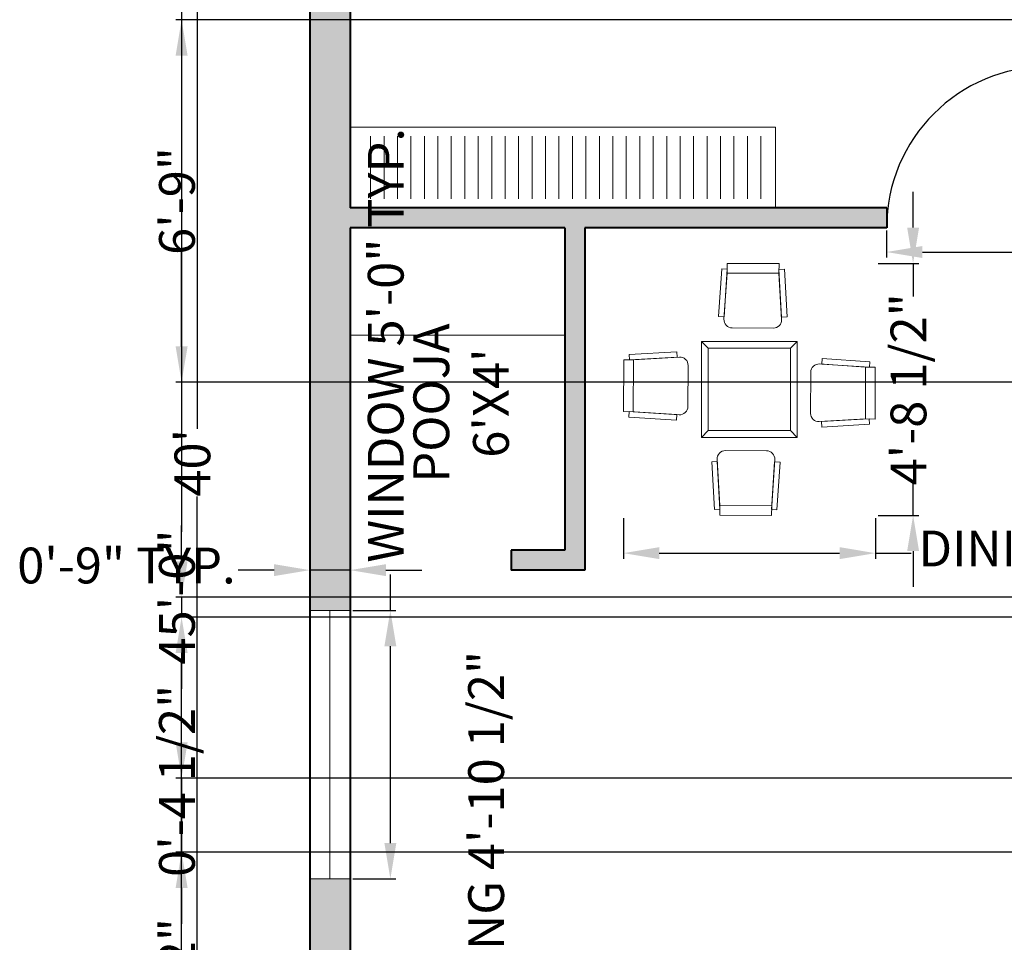
# Model space of a CAD drawing. Units: inches. Extents: x 2138 to 3265, y 2149 to 3392.
# Tile 3 of 13: x 2143 to 2363, y 2382 to 2589. Entities that reach past the tile are written whole.
import ezdxf

# ---------------------------------------------------------------- set-up
doc = ezdxf.new("R2010")
doc.units = ezdxf.units.IN
for name, color, linetype, lineweight in [('A-ANNO-DIMS', 2, 'Continuous', 18), ('A-AREA-IDEN', 7, 'Continuous', 18), ('A-DOOR', 22, 'Continuous', 25), ('A-FLOR-CASE', 30, 'Continuous', 20), ('A-FLOR-CASE-PATT', 251, 'Continuous', 13), ('A-FURN', 8, 'Continuous', 18), ('A-GLAZ', 150, 'Continuous', 18), ('A-WALL', 7, 'Continuous', 40), ('A-WALL-PATT', 142, 'Continuous', 13)]:
    doc.layers.add(name, color=color, linetype=linetype, lineweight=lineweight)
doc.styles.get("Standard").update_dxf_attribs({"font": 'arial.ttf'})
doc.dimstyles.new('ISO-25', dxfattribs={"dimtxt": 8, "dimasz": 8, "dimexe": 1.25, "dimexo": 0.625, "dimtad": 0, "dimdec": 1, "dimlunit": 4, "dimtxsty": 'Standard', "dimcen": 2.5, "dimadec": 0, "dimazin": 0, "dimtfac": 1, "dimtdec": 1, "dimtmove": 0, "dimatfit": 3, "dimfxl": 1, "dimarcsym": 0})

# ---------------------------------------------------------------- blocks, each defined once
blk = doc.blocks.new('db')
for p, q in [((2724.14, 2649.34), (2722.17, 2651.31)), ((2749.73, 2651.31), (2747.76, 2649.34)), ((2724.14, 2625.72), (2722.17, 2623.75)), ((2749.73, 2623.75), (2747.76, 2625.72))]:
    blk.add_line(p, q)
for points in [[(2728.69, 2658.35), (2727.1, 2658.45), (2728.01, 2672.17), (2729.59, 2672.07)], [(2729.53, 2670.94), (2729.55, 2673.73), (2744.47, 2673.66), (2744.46, 2670.87)], [(2745.19, 2658.27), (2746.78, 2658.36), (2746, 2672.08), (2744.41, 2672)], [(2722.17, 2651.31), (2749.73, 2651.31), (2749.73, 2623.75), (2722.17, 2623.75)], [(2724.14, 2649.34), (2747.76, 2649.34), (2747.76, 2625.72), (2724.14, 2625.72)], [(2715.21, 2646.77), (2715.13, 2648.36), (2701.4, 2647.58), (2701.49, 2645.99)], [(2756.76, 2644.8), (2756.86, 2646.38), (2770.59, 2645.48), (2770.48, 2643.89)], [(2702.54, 2631.12), (2699.75, 2631.13), (2699.82, 2646.06), (2702.61, 2646.04)], [(2769.36, 2643.95), (2772.15, 2643.94), (2772.08, 2629.01), (2769.29, 2629.02)], [(2715.14, 2630.27), (2715.03, 2628.68), (2701.31, 2629.59), (2701.42, 2631.18)], [(2756.68, 2628.29), (2756.77, 2626.7), (2770.5, 2627.49), (2770.41, 2629.07)], [(2726.71, 2616.8), (2725.12, 2616.71), (2725.9, 2602.98), (2727.49, 2603.07)], [(2743.21, 2616.72), (2744.8, 2616.62), (2743.89, 2602.9), (2742.3, 2603)], [(2742.37, 2604.12), (2742.35, 2601.34), (2727.43, 2601.41), (2727.44, 2604.19)]]:
    blk.add_lwpolyline(points, close=True)
for points in [[(2745.22, 2657.63, -0.431982), (2742.85, 2655.13), (2731, 2655.19, -0.431982), (2728.65, 2657.7), (2729.53, 2670.94), (2744.46, 2670.87)], [(2715.86, 2646.8, -0.431982), (2718.35, 2644.43), (2718.29, 2632.58, -0.431982), (2715.78, 2630.23), (2702.54, 2631.12), (2702.61, 2646.04)], [(2756.04, 2628.26, -0.431982), (2753.55, 2630.63), (2753.6, 2642.49, -0.431982), (2756.12, 2644.83), (2769.36, 2643.95), (2769.29, 2629.02)], [(2726.68, 2617.44, -0.431982), (2729.05, 2619.93), (2740.9, 2619.88, -0.431982), (2743.25, 2617.36), (2742.37, 2604.12), (2727.44, 2604.19)]]:
    blk.add_lwpolyline(points, format="xyb", close=True)
blk = doc.blocks.new('door')
blk.add_lwpolyline([(2064.92, 2369.1), (2066.69, 2369.1), (2066.69, 2393.11), (2064.92, 2393.11)], close=True)
blk.add_arc((2066.69, 2369.1), 24.02, 90, 180)
blk = doc.blocks.new('*D19')
at = {"layer": 'A-ANNO-DIMS', "color": 0, "lineweight": -2, "transparency": 16777216}
for p, q in [((2206.9, 2729.66), (2181.05, 2729.66)), ((2182.3, 2721.66), (2182.3, 2497.24)), ((2182.3, 2257.66), (2182.3, 2482.09)), ((2206.9, 2249.66), (2181.05, 2249.66))]:
    blk.add_line(p, q, dxfattribs=at)
at = {"layer": 'A-ANNO-DIMS', "color": 0, "transparency": 16777216}
for points in [[(2180.97, 2721.66), (2183.63, 2721.66), (2182.3, 2729.66)], [(2180.97, 2257.66), (2183.63, 2257.66), (2182.3, 2249.66)]]:
    blk.add_solid(points, dxfattribs=at)
at = {"layer": 'Defpoints', "color": 0, "transparency": 16777216}
for p in [(2207.53, 2729.66), (2182.3, 2249.66), (2207.53, 2249.66)]:
    blk.add_point(p, dxfattribs=at)
at = {"layer": 'A-ANNO-DIMS', "color": 0, "transparency": 16777216, "insert": (2182.3, 2489.66), "char_height": 8, "attachment_point": 5, "rotation": 90}
blk.add_mtext("40'", dxfattribs=at)
blk = doc.blocks.new('GLAZ-SASH-60IN')
for p, q in [((0, 9), (0, 0)), ((60, 9), (60, 0)), ((0, 4.5), (60, 4.5))]:
    blk.add_line(p, q)
blk = doc.blocks.new('*D23')
at = {"layer": 'A-ANNO-DIMS', "color": 0, "lineweight": -2, "transparency": 16777216}
for p, q in [((2225.53, 2456.66), (2225.53, 2464.66)), ((2217.15, 2456.66), (2226.78, 2456.66)), ((2225.53, 2404.66), (2225.53, 2448.66)), ((2217.15, 2396.66), (2226.78, 2396.66))]:
    blk.add_line(p, q, dxfattribs=at)
at = {"layer": 'A-ANNO-DIMS', "color": 0, "transparency": 16777216}
for points in [[(2224.2, 2448.66), (2226.86, 2448.66), (2225.53, 2456.66)], [(2224.2, 2404.66), (2226.86, 2404.66), (2225.53, 2396.66)]]:
    blk.add_solid(points, dxfattribs=at)
at = {"layer": 'Defpoints', "color": 0, "transparency": 16777216}
for p in [(2216.53, 2456.66), (2225.53, 2456.66), (2216.53, 2396.66)]:
    blk.add_point(p, dxfattribs=at)
at = {"layer": 'A-ANNO-DIMS', "color": 0, "transparency": 16777216, "insert": (2225.53, 2515.9), "char_height": 8, "attachment_point": 5, "rotation": 90}
blk.add_mtext('WINDOW 5\'-0" TYP.', dxfattribs=at)
blk = doc.blocks.new('*D24')
at = {"layer": 'A-ANNO-DIMS', "color": 0, "lineweight": -2, "transparency": 16777216}
for p, q in [((2199.53, 2465.66), (2191.53, 2465.66)), ((2207.53, 2457.29), (2207.53, 2466.91)), ((2216.53, 2465.66), (2207.53, 2465.66)), ((2216.53, 2457.29), (2216.53, 2466.91)), ((2224.53, 2465.66), (2232.53, 2465.66))]:
    blk.add_line(p, q, dxfattribs=at)
at = {"layer": 'A-ANNO-DIMS', "color": 0, "transparency": 16777216}
for points in [[(2199.53, 2466.99), (2199.53, 2464.33), (2207.53, 2465.66)], [(2224.53, 2466.99), (2224.53, 2464.33), (2216.53, 2465.66)]]:
    blk.add_solid(points, dxfattribs=at)
at = {"layer": 'Defpoints', "color": 0, "transparency": 16777216}
for p in [(2207.53, 2465.66), (2207.53, 2456.66), (2216.53, 2456.66)]:
    blk.add_point(p, dxfattribs=at)
at = {"layer": 'A-ANNO-DIMS', "color": 0, "transparency": 16777216, "insert": (2166.52, 2465.66), "char_height": 8, "attachment_point": 5}
blk.add_mtext('0\'-9" TYP.', dxfattribs=at)
blk = doc.blocks.new('*D27')
at = {"layer": 'A-ANNO-DIMS', "color": 0, "lineweight": -2, "transparency": 16777216}
for p, q in [((2336.48, 2541.54), (2336.48, 2535.5)), ((2372.53, 2541.54), (2372.53, 2535.5)), ((2344.48, 2536.75), (2364.53, 2536.75)), ((2372.53, 2536.75), (2380.53, 2536.75))]:
    blk.add_line(p, q, dxfattribs=at)
at = {"layer": 'A-ANNO-DIMS', "color": 0, "transparency": 16777216}
for points in [[(2344.48, 2538.09), (2344.48, 2535.42), (2336.48, 2536.75)], [(2364.53, 2538.09), (2364.53, 2535.42), (2372.53, 2536.75)]]:
    blk.add_solid(points, dxfattribs=at)
at = {"layer": 'Defpoints', "color": 0, "transparency": 16777216}
for p in [(2336.48, 2542.16), (2372.53, 2542.16), (2372.53, 2536.75)]:
    blk.add_point(p, dxfattribs=at)
at = {"layer": 'A-ANNO-DIMS', "color": 0, "transparency": 16777216, "insert": (2442.58, 2536.75), "char_height": 8, "attachment_point": 5}
blk.add_mtext('ROOM DOOR 3\'-0" TYP.', dxfattribs=at)
blk = doc.blocks.new('*D37')
at = {"layer": 'A-ANNO-DIMS', "color": 0, "lineweight": -2, "transparency": 16777216}
for p, q in [((2277.64, 2477.28), (2277.64, 2468.21)), ((2333.96, 2477.28), (2333.96, 2468.21)), ((2285.64, 2469.46), (2325.96, 2469.46)), ((2333.96, 2469.46), (2341.96, 2469.46))]:
    blk.add_line(p, q, dxfattribs=at)
at = {"layer": 'A-ANNO-DIMS', "color": 0, "transparency": 16777216}
for points in [[(2285.64, 2470.8), (2285.64, 2468.13), (2277.64, 2469.46)], [(2325.96, 2470.8), (2325.96, 2468.13), (2333.96, 2469.46)]]:
    blk.add_solid(points, dxfattribs=at)
at = {"layer": 'Defpoints', "color": 0, "transparency": 16777216}
for p in [(2277.64, 2477.91), (2333.96, 2477.91), (2333.96, 2469.46)]:
    blk.add_point(p, dxfattribs=at)
at = {"layer": 'A-ANNO-DIMS', "color": 0, "transparency": 16777216, "insert": (2395.87, 2469.46), "char_height": 8, "attachment_point": 5}
blk.add_mtext('DINING SET 4\'-8 1/2"', dxfattribs=at)
blk = doc.blocks.new('*D38')
at = {"layer": 'A-ANNO-DIMS', "color": 0, "lineweight": -2, "transparency": 16777216}
for p, q in [((2342.4, 2542.22), (2342.4, 2550.22)), ((2334.58, 2534.22), (2343.65, 2534.22)), ((2342.4, 2534.22), (2342.4, 2526.81)), ((2342.4, 2477.91), (2342.4, 2485.33)), ((2334.58, 2477.91), (2343.65, 2477.91)), ((2342.4, 2469.91), (2342.4, 2461.91))]:
    blk.add_line(p, q, dxfattribs=at)
at = {"layer": 'A-ANNO-DIMS', "color": 0, "transparency": 16777216}
for points in [[(2341.07, 2542.22), (2343.74, 2542.22), (2342.4, 2534.22)], [(2341.07, 2469.91), (2343.74, 2469.91), (2342.4, 2477.91)]]:
    blk.add_solid(points, dxfattribs=at)
at = {"layer": 'Defpoints', "color": 0, "transparency": 16777216}
for p in [(2333.96, 2534.22), (2342.4, 2534.22), (2333.96, 2477.91)]:
    blk.add_point(p, dxfattribs=at)
at = {"layer": 'A-ANNO-DIMS', "color": 0, "transparency": 16777216, "insert": (2342.4, 2506.07), "char_height": 8, "attachment_point": 5, "rotation": 90}
blk.add_mtext('4\'-8 1/2"', dxfattribs=at)
blk = doc.blocks.new('*D41')
at = {"layer": 'A-ANNO-DIMS', "color": 0, "lineweight": -2, "transparency": 16777216}
for p, q in [((2247.97, 2341.8), (2247.97, 2349.8)), ((2239.81, 2341.8), (2249.22, 2341.8)), ((2247.97, 2291.25), (2247.97, 2333.8)), ((2239.81, 2283.25), (2249.22, 2283.25))]:
    blk.add_line(p, q, dxfattribs=at)
at = {"layer": 'A-ANNO-DIMS', "color": 0, "transparency": 16777216}
for points in [[(2246.64, 2333.8), (2249.3, 2333.8), (2247.97, 2341.8)], [(2246.64, 2291.25), (2249.3, 2291.25), (2247.97, 2283.25)]]:
    blk.add_solid(points, dxfattribs=at)
at = {"layer": 'Defpoints', "color": 0, "transparency": 16777216}
for p in [(2239.19, 2341.8), (2247.97, 2341.8), (2239.19, 2283.25)]:
    blk.add_point(p, dxfattribs=at)
at = {"layer": 'A-ANNO-DIMS', "color": 0, "transparency": 16777216, "insert": (2247.97, 2399.55), "char_height": 8, "attachment_point": 5, "rotation": 90}
blk.add_mtext('SEATING 4\'-10 1/2"', dxfattribs=at)
blk = doc.blocks.new('*D51')
at = {"layer": 'A-ANNO-DIMS', "color": 0, "lineweight": -2, "transparency": 16777216}
for p, q in [((2206.9, 2729.66), (2177.6, 2729.66)), ((2178.85, 2721.66), (2178.85, 2474.19)), ((2178.85, 2197.66), (2178.85, 2445.13)), ((2206.9, 2189.66), (2177.6, 2189.66))]:
    blk.add_line(p, q, dxfattribs=at)
at = {"layer": 'A-ANNO-DIMS', "color": 0, "transparency": 16777216}
for points in [[(2177.52, 2721.66), (2180.19, 2721.66), (2178.85, 2729.66)], [(2177.52, 2197.66), (2180.19, 2197.66), (2178.85, 2189.66)]]:
    blk.add_solid(points, dxfattribs=at)
at = {"layer": 'Defpoints', "color": 0, "transparency": 16777216}
for p in [(2178.85, 2729.66), (2207.53, 2729.66), (2207.53, 2189.66)]:
    blk.add_point(p, dxfattribs=at)
at = {"layer": 'A-ANNO-DIMS', "color": 0, "transparency": 16777216, "insert": (2178.85, 2459.66), "char_height": 8, "attachment_point": 5, "rotation": 90}
blk.add_mtext('45\'-0"', dxfattribs=at)
blk = doc.blocks.new('*D53')
at = {"layer": 'A-ANNO-DIMS', "color": 0, "lineweight": -2, "transparency": 16777216}
for p, q in [((2178.85, 2467.66), (2178.85, 2475.66)), ((2497.9, 2459.66), (2177.6, 2459.66)), ((2178.85, 2459.66), (2178.85, 2455.16)), ((2497.9, 2455.16), (2177.6, 2455.16)), ((2178.85, 2447.16), (2178.85, 2439.16))]:
    blk.add_line(p, q, dxfattribs=at)
at = {"layer": 'A-ANNO-DIMS', "color": 0, "transparency": 16777216}
for points in [[(2177.52, 2467.66), (2180.19, 2467.66), (2178.85, 2459.66)], [(2177.52, 2447.16), (2180.19, 2447.16), (2178.85, 2455.16)]]:
    blk.add_solid(points, dxfattribs=at)
at = {"layer": 'Defpoints', "color": 0, "transparency": 16777216}
for p in [(2498.53, 2459.66), (2178.85, 2455.16), (2498.53, 2455.16)]:
    blk.add_point(p, dxfattribs=at)
at = {"layer": 'A-ANNO-DIMS', "color": 0, "transparency": 16777216, "insert": (2178.85, 2418.58), "char_height": 8, "attachment_point": 5, "rotation": 90}
blk.add_mtext('0\'-4 1/2"', dxfattribs=at)
blk = doc.blocks.new('*D55')
at = {"layer": 'A-ANNO-DIMS', "color": 0, "lineweight": -2, "transparency": 16777216}
for p, q in [((2455.9, 2588.66), (2177.6, 2588.66)), ((2178.85, 2580.66), (2178.85, 2559.44)), ((2178.85, 2515.66), (2178.85, 2536.88)), ((2455.9, 2507.66), (2177.6, 2507.66))]:
    blk.add_line(p, q, dxfattribs=at)
at = {"layer": 'A-ANNO-DIMS', "color": 0, "transparency": 16777216}
for points in [[(2177.52, 2580.66), (2180.19, 2580.66), (2178.85, 2588.66)], [(2177.52, 2515.66), (2180.19, 2515.66), (2178.85, 2507.66)]]:
    blk.add_solid(points, dxfattribs=at)
at = {"layer": 'Defpoints', "color": 0, "transparency": 16777216}
for p in [(2456.53, 2588.66), (2178.85, 2507.66), (2456.53, 2507.66)]:
    blk.add_point(p, dxfattribs=at)
at = {"layer": 'A-ANNO-DIMS', "color": 0, "transparency": 16777216, "insert": (2178.85, 2548.16), "char_height": 8, "attachment_point": 5, "rotation": 90}
blk.add_mtext('6\'-9"', dxfattribs=at)
blk = doc.blocks.new('*D60')
at = {"layer": 'A-ANNO-DIMS', "color": 0, "lineweight": -2, "transparency": 16777216}
for p, q in [((2178.85, 2427.16), (2178.85, 2435.16)), ((2493.4, 2419.16), (2177.6, 2419.16)), ((2178.85, 2419.16), (2178.85, 2402.66)), ((2493.4, 2402.66), (2177.6, 2402.66)), ((2178.85, 2394.66), (2178.85, 2386.66))]:
    blk.add_line(p, q, dxfattribs=at)
at = {"layer": 'A-ANNO-DIMS', "color": 0, "transparency": 16777216}
for points in [[(2177.52, 2427.16), (2180.19, 2427.16), (2178.85, 2419.16)], [(2177.52, 2394.66), (2180.19, 2394.66), (2178.85, 2402.66)]]:
    blk.add_solid(points, dxfattribs=at)
at = {"layer": 'Defpoints', "color": 0, "transparency": 16777216}
for p in [(2494.03, 2419.16), (2178.85, 2402.66), (2494.03, 2402.66)]:
    blk.add_point(p, dxfattribs=at)
at = {"layer": 'A-ANNO-DIMS', "color": 0, "transparency": 16777216, "insert": (2178.85, 2366.46), "char_height": 8, "attachment_point": 5, "rotation": 90}
blk.add_mtext('1\'-4 1/2"', dxfattribs=at)

msp = doc.modelspace()

# ---------------------------------------------------------------- hatches: boundary and pattern name
at = {"layer": 'A-FLOR-CASE-PATT'}
h = msp.add_hatch(dxfattribs=at)
h.set_pattern_fill('ANSI31', color=256, scale=0.94791, angle=45, style=0)
h.paths.add_polyline_path([(2219.6, 2548.66), (2309.89, 2548.66), (2309.89, 2562.66), (2219.6, 2562.66)])
at = {"layer": 'A-WALL-PATT'}
h = msp.add_hatch(color=256, dxfattribs=at)
h.dxf.hatch_style = 1
h.paths.add_polyline_path([(2270.53, 2729.66), (2207.53, 2729.66), (2207.53, 2663.66), (2216.53, 2663.66), (2216.53, 2720.66), (2270.53, 2720.66)])
h.paths.add_polyline_path([(2484.36, 2729.66), (2330.53, 2729.66), (2330.53, 2720.66), (2384.53, 2720.66), (2384.53, 2546.66), (2372.53, 2546.66), (2372.53, 2542.16), (2389.03, 2542.16), (2389.03, 2720.66), (2484.36, 2720.66)])
h.paths.add_polyline_path([(2591.53, 2729.66), (2544.36, 2729.66), (2544.36, 2720.66), (2582.53, 2720.66), (2582.53, 2684.66), (2591.53, 2684.66)])
h.paths.add_polyline_path([(2591.53, 2624.66), (2582.53, 2624.66), (2582.53, 2588.66), (2456.53, 2588.66), (2456.53, 2584.16), (2582.53, 2584.16), (2582.53, 2512.16), (2456.53, 2512.16), (2456.53, 2507.66), (2494.03, 2507.66), (2494.03, 2501.66), (2498.53, 2501.66), (2498.53, 2507.66), (2582.53, 2507.66), (2582.53, 2495.66), (2591.53, 2495.66)])
h.paths.add_polyline_path([(2591.53, 2471.66), (2582.53, 2471.66), (2582.53, 2459.66), (2498.53, 2459.66), (2498.53, 2471.66), (2497.72, 2471.66, -0.030629), (2494.03, 2471.44), (2494.03, 2459.66), (2431.08, 2459.66, -0.013128), (2431.03, 2457.77), (2431.03, 2455.16), (2494.03, 2455.16), (2494.03, 2449.16), (2498.53, 2449.16), (2498.53, 2455.16), (2582.53, 2455.16), (2582.53, 2443.16), (2591.53, 2443.16)])
h.paths.add_polyline_path([(2591.53, 2419.16), (2582.53, 2419.16), (2582.53, 2407.16), (2498.53, 2407.16), (2498.53, 2419.16), (2497.72, 2419.16, -0.030629), (2494.03, 2418.94), (2494.03, 2402.66), (2582.53, 2402.66), (2582.53, 2360.66), (2591.53, 2360.66)])
h.paths.add_polyline_path([(2591.53, 2300.66), (2582.53, 2300.66), (2582.53, 2258.66), (2515.78, 2258.66), (2515.78, 2249.66), (2591.53, 2249.66)])
h.paths.add_polyline_path([(2455.78, 2258.66), (2389.03, 2258.66), (2389.03, 2455.16), (2395.03, 2455.16), (2395.03, 2459.66), (2384.53, 2459.66), (2384.53, 2258.66), (2375.53, 2258.66), (2375.53, 2249.66), (2455.78, 2249.66)])
h.paths.add_polyline_path([(2315.53, 2253.24), (2315.53, 2258.66), (2296.03, 2258.66), (2296.03, 2249.66), (2315.53, 2249.66)])
h.paths.add_polyline_path([(2236.03, 2258.66), (2216.53, 2258.66), (2216.53, 2290.16), (2207.53, 2290.16), (2207.53, 2249.66), (2236.03, 2249.66)])
h.paths.add_polyline_path([(2216.53, 2396.66), (2207.53, 2396.66), (2207.53, 2350.16), (2216.53, 2350.16)])
h.paths.add_polyline_path([(2216.53, 2603.66), (2207.53, 2603.66), (2207.53, 2456.66), (2216.53, 2456.66), (2216.53, 2542.16), (2264.53, 2542.16), (2264.53, 2470.16), (2252.53, 2470.16), (2252.53, 2465.66), (2269.03, 2465.66), (2269.03, 2542.16), (2336.48, 2542.16, -0.013128), (2336.53, 2544.05), (2336.53, 2546.66), (2216.53, 2546.66)])

# ---------------------------------------------------------------- linework, layer by layer
at = {"layer": 'A-FLOR-CASE'}
for p, q in [((2311.64, 2564.66), (2216.53, 2564.66)), ((2311.64, 2564.66), (2311.64, 2546.66)), ((2264.53, 2518.16), (2216.53, 2518.16))]:
    msp.add_line(p, q, dxfattribs=at)
at = {"layer": 'A-GLAZ'}
msp.add_lwpolyline([(2207.53, 2456.66), (2216.53, 2456.66), (2216.53, 2396.66), (2207.53, 2396.66)], close=True, dxfattribs=at)
at = {"layer": 'A-WALL'}
for p, q in [((2207.53, 2729.66), (2207.53, 2189.66)), ((2216.53, 2720.66), (2216.53, 2546.66)), ((2336.53, 2546.66), (2216.53, 2546.66)), ((2336.53, 2546.66), (2336.53, 2542.16)), ((2264.53, 2542.16), (2216.53, 2542.16)), ((2216.53, 2542.16), (2216.53, 2456.66)), ((2264.53, 2542.16), (2264.53, 2470.16)), ((2269.03, 2542.16), (2269.03, 2465.66)), ((2336.53, 2542.16), (2269.03, 2542.16)), ((2264.53, 2470.16), (2252.53, 2470.16)), ((2252.53, 2470.16), (2252.53, 2465.66)), ((2269.03, 2465.66), (2252.53, 2465.66)), ((2216.53, 2456.66), (2216.53, 2258.66))]:
    msp.add_line(p, q, dxfattribs=at)

# ---------------------------------------------------------------- block references
at = {"layer": 'A-DOOR', "xscale": 1.501085369916538, "yscale": 1.501085369916538, "zscale": 1.501085369916538}
msp.add_blockref('door', (-729.75, -1014.05), dxfattribs=at)
at = {"layer": 'A-FURN', "xscale": 0.777867820292987, "yscale": 0.777867820292987, "zscale": 0.777867820292987}
msp.add_blockref('db', (177.59, 454.41), dxfattribs=at)
at = {"layer": 'A-GLAZ', "rotation": 89.9999999999994}
msp.add_blockref('GLAZ-SASH-60IN', (2216.53, 2396.66), dxfattribs=at)

# ---------------------------------------------------------------- texts
at = {"layer": 'A-AREA-IDEN', "insert": (2230.68, 2464.49), "char_height": 8, "attachment_point": 1, "rotation": 90}
msp.add_mtext_dynamic_manual_height_columns("\\pxqc;POOJA\\P6'X4'", width=77.0226, gutter_width=12.5, heights=[0], dxfattribs=at)

# ---------------------------------------------------------------- dimensions: what is measured, and where the dimension line sits
at = {"layer": 'A-ANNO-DIMS'}
for base, p1, p2, override, picture, middle in [((2178.85, 2729.66), (2207.53, 2189.66), (2207.53, 2729.66), {"dimdec": 1, "dimlfac": 1, "dimrnd": 0, "dimzin": 1, "dimdsep": 46, "dimlunit": 4, "dimfrac": 2}, '*D51', (2178.85, 2459.66)), ((2182.3, 2249.66), (2207.53, 2729.66), (2207.53, 2249.66), {"dimclrd": 0, "dimclre": 0, "dimclrt": 0}, '*D19', (2182.3, 2489.66)), ((2178.85, 2507.66), (2456.53, 2588.66), (2456.53, 2507.66), {"dimdec": 1, "dimlfac": 1, "dimrnd": 0, "dimzin": 1, "dimdsep": 46, "dimlunit": 4, "dimfrac": 2}, '*D55', (2178.85, 2548.16)), ((2342.4, 2534.22), (2333.96, 2477.91), (2333.96, 2534.22), {"dimdec": 1, "dimlfac": 1, "dimrnd": 0, "dimzin": 1, "dimdsep": 46, "dimlunit": 4, "dimfrac": 2}, '*D38', (2342.4, 2506.07)), ((2178.85, 2455.16), (2498.53, 2459.66), (2498.53, 2455.16), {"dimdec": 1, "dimlfac": 1, "dimrnd": 0, "dimzin": 1, "dimdsep": 46, "dimlunit": 4, "dimfrac": 2}, '*D53', (2178.85, 2418.58)), ((2178.85, 2402.66), (2494.03, 2419.16), (2494.03, 2402.66), {"dimdec": 1, "dimlfac": 1, "dimrnd": 0, "dimzin": 1, "dimdsep": 46, "dimlunit": 4, "dimfrac": 2}, '*D60', (2178.85, 2366.46))]:
    dim = msp.add_linear_dim(base=base, p1=p1, p2=p2, angle=90, dimstyle='ISO-25', override=override, dxfattribs=at)
    dim.commit()
    dim.dimension.update_dxf_attribs({"geometry": picture, "text_midpoint": middle})
for base, p1, p2, angle, text, picture, middle in [((2225.53, 2456.66), (2216.53, 2396.66), (2216.53, 2456.66), 90, 'WINDOW <> TYP.', '*D23', (2225.53, 2515.9)), ((2207.53, 2465.66), (2216.53, 2456.66), (2207.53, 2456.66), 180, '<> TYP.', '*D24', (2166.52, 2465.66)), ((2247.9691, 2341.7994), (2239.187, 2283.2518), (2239.187, 2341.7994), 90, 'SEATING <>', '*D41', (2247.9691, 2399.5485))]:
    dim = msp.add_linear_dim(base=base, p1=p1, p2=p2, angle=angle, text=text, dimstyle='ISO-25', override={"dimdec": 1, "dimlfac": 1, "dimrnd": 0, "dimzin": 1, "dimdsep": 46, "dimlunit": 4, "dimfrac": 2}, dxfattribs=at)
    dim.commit()
    dim.dimension.update_dxf_attribs({"geometry": picture, "text_midpoint": middle})
for base, p1, p2, text, picture, middle in [((2372.5295, 2536.7541), (2336.4798, 2542.1616), (2372.5295, 2542.1616), 'ROOM DOOR <> TYP.', '*D27', (2442.5815, 2536.7541)), ((2333.96, 2469.46), (2277.64, 2477.91), (2333.96, 2477.91), 'DINING SET <>', '*D37', (2395.87, 2469.46))]:
    dim = msp.add_linear_dim(base=base, p1=p1, p2=p2, text=text, dimstyle='ISO-25', override={"dimdec": 1, "dimlfac": 1, "dimrnd": 0, "dimzin": 1, "dimdsep": 46, "dimlunit": 4, "dimfrac": 2}, dxfattribs=at)
    dim.commit()
    dim.dimension.update_dxf_attribs({"geometry": picture, "text_midpoint": middle})

doc.saveas('drawing.dxf')
